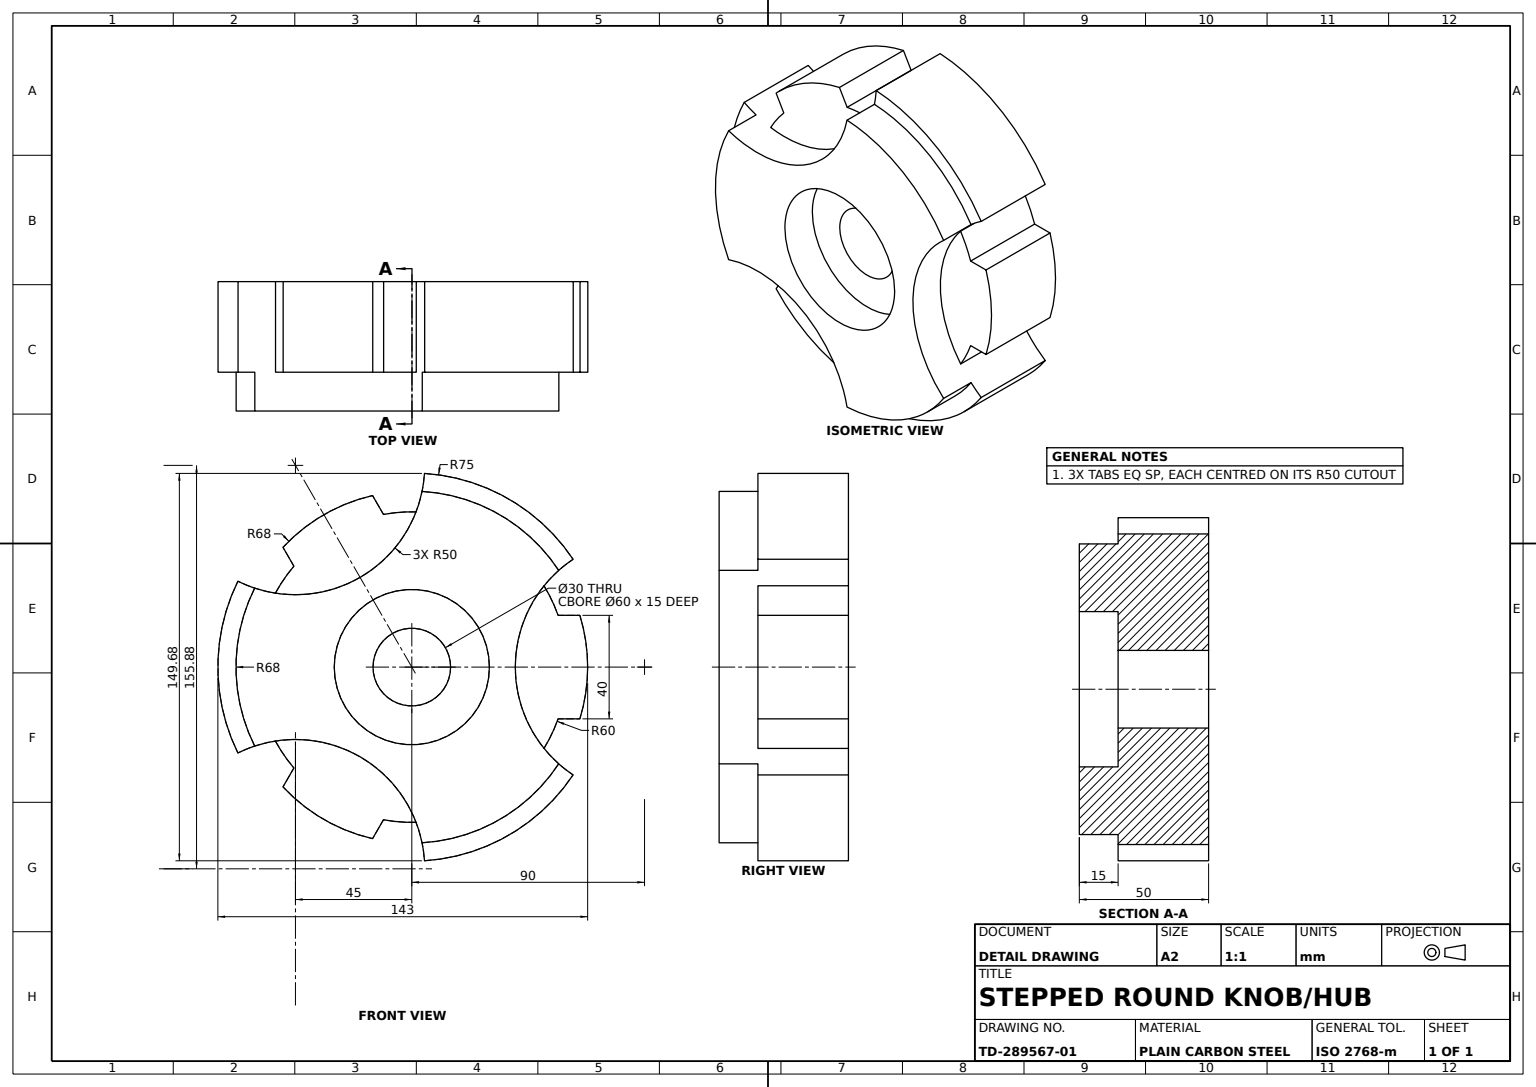
from build123d import *

# Parameters (mm, degrees)
BASE_BODY_35MM_DEPTH          = 35
THREE_LOBE_PROFILE_35MM_DEPTH = 35
RAISED_HUB_15MM_DEPTH         = 15
COUNTERBORE_SKETCH_60_R       = 30
COUNTERBORE_60X15_DEPTH       = 15
BORE_SKETCH_30_R              = 15
THROUGH_BORE_30_DEPTH         = 35


with BuildPart() as part:
    # Base Profile Sketch → Base Body 35mm (new body)
    with BuildSketch(Plane(origin=(0, 0, 0), x_dir=(1, 0, 0), z_dir=(0, 1, 0))):
        with BuildLine():
            ThreePointArc((-41.666435185, 62.361111111), (-64.951905284, 37.5), (-74.839524023, 4.903635799))
            ThreePointArc((-74.839524023, 4.903635799), (-34.641016151, -20), (-33.173088838, -67.264746911))
            ThreePointArc((-33.173088838, -67.264746911), (0, -75), (33.173088838, -67.264746911))
            ThreePointArc((33.173088838, -67.264746911), (34.641016151, -20), (74.839524023, 4.903635799))
            ThreePointArc((74.839524023, 4.903635799), (64.951905284, 37.5), (41.666435185, 62.361111111))
            ThreePointArc((41.666435185, 62.361111111), (0, 40), (-41.666435185, 62.361111111))
        make_face()
    extrude(amount=BASE_BODY_35MM_DEPTH)

    # Lobe Profile Sketch → Three-Lobe Profile 35mm (add)
    with BuildSketch(Plane.XZ):
        with BuildLine():
            Line((20, -56.568542495), (20, -64.992307237))
            ThreePointArc((20, -64.992307237), (0, -68), (-20, -64.992307237))
            Line((-20, -64.992307237), (-20, -56.568542495))
            ThreePointArc((-20, -56.568542495), (-51.961524227, -30), (-58.989794856, 10.963763172))
            Line((-58.989794856, 10.963763172), (-66.284989118, 15.175645543))
            ThreePointArc((-66.284989118, 15.175645543), (-58.889727457, 34), (-46.284989118, 49.816661694))
            Line((-46.284989118, 49.816661694), (-38.989794856, 45.604779323))
            ThreePointArc((-38.989794856, 45.604779323), (0, 60), (38.989794856, 45.604779323))
            Line((38.989794856, 45.604779323), (46.284989118, 49.816661694))
            ThreePointArc((46.284989118, 49.816661694), (58.889727457, 34), (66.284989118, 15.175645543))
            Line((66.284989118, 15.175645543), (58.989794856, 10.963763172))
            ThreePointArc((58.989794856, 10.963763172), (51.961524227, -30), (20, -56.568542495))
        make_face()
    extrude(amount=-THREE_LOBE_PROFILE_35MM_DEPTH)

    # Hub Profile Sketch → Raised Hub 15mm (add)
    with BuildSketch(Plane(origin=(0, 35, 0), x_dir=(1, 0, 0), z_dir=(0, 1, 0))):
        with BuildLine():
            ThreePointArc((-37.386628626, 56.8), (-58.889727457, 34), (-67.883557248, 3.977770152))
            ThreePointArc((-67.883557248, 3.977770152), (-34.641016151, -20), (-30.496928622, -60.777770152))
            ThreePointArc((-30.496928622, -60.777770152), (0, -68), (30.496928622, -60.777770152))
            ThreePointArc((30.496928622, -60.777770152), (34.641016151, -20), (67.883557248, 3.977770152))
            ThreePointArc((67.883557248, 3.977770152), (58.889727457, 34), (37.386628626, 56.8))
            ThreePointArc((37.386628626, 56.8), (0, 40), (-37.386628626, 56.8))
        make_face()
    extrude(amount=RAISED_HUB_15MM_DEPTH)

    # Counterbore Sketch Ø60 → Counterbore Ø60x15 (cut)
    with BuildSketch(Plane(origin=(0, 50, 0), x_dir=(1, 0, 0), z_dir=(0, 1, 0))):
        with Locations(Location((0, 0, 0), (0, 0, 270))):
            Circle(COUNTERBORE_SKETCH_60_R)
    extrude(amount=-COUNTERBORE_60X15_DEPTH, mode=Mode.SUBTRACT)

    # Bore Sketch Ø30 → Through Bore Ø30 (cut)
    with BuildSketch(Plane(origin=(0, 35, 0), x_dir=(1, 0, 0), z_dir=(0, 1, 0))):
        with Locations(Location((0, 0, 0), (0, 0, 270))):
            Circle(BORE_SKETCH_30_R)
    extrude(amount=-THROUGH_BORE_30_DEPTH, mode=Mode.SUBTRACT)


solid = part.part
